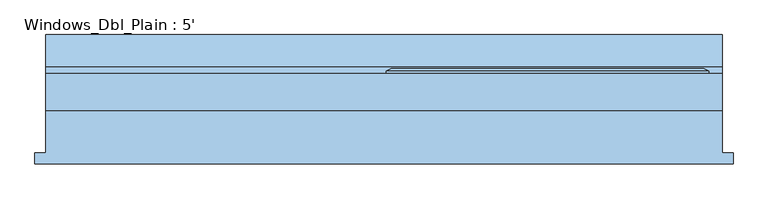
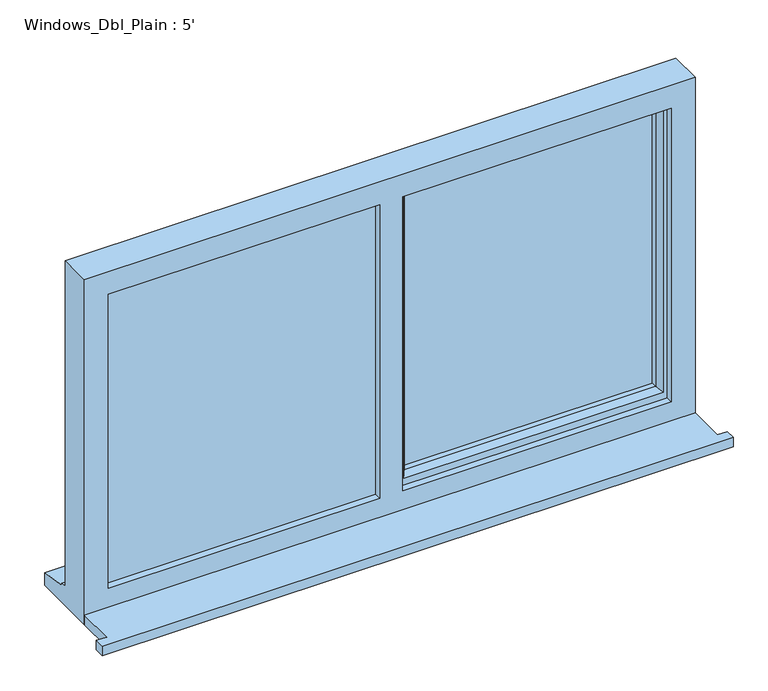
"""IFC4 building model written with IfcOpenShell, lengths in millimetres: window geometry, Windows_Dbl_Plain : 5'."""

from ifc_helpers import new_model, si_unit, frame, origin, place, context, project, spatial, polyline, outline, extrude, faceted_brep, source, transform, mapped, element, save


def windows_dbl_plain_5_e9a2d570(model_context):
    return source(origin(), model_context, "Body", "SolidModel", [
        extrude(outline(polyline([(-1072.0, -130.8434322), (-1072.0, -105.8434322), (-1047.0, -105.8434322), (-1047.0, -10.2434322), (477.0, -10.2434322), (477.0, -105.8434322), (502.0, -105.8434322), (502.0, -130.8434322), (-1072.0, -130.8434322)])), frame((0.0, 0.0, 1200.0), z_axis=(0.0, 0.0, 1.0), x_axis=(1.0, 0.0, 0.0)), (0.0, 0.0, 1.0), 25.0),
        faceted_brep([(-280.0, 72.7565678, 2080.0), (-280.0, 78.5300705, 2080.0), (-280.0, 78.5300705, 1253.0), (-280.0, 72.7565678, 1253.0), (-270.0, 7.7565678, 2070.0), (-270.0, 72.7565678, 2070.0), (-270.0, 72.7565678, 1263.0), (-270.0, 7.7565678, 1263.0), (-230.0, 22.2494677, 2030.0), (-240.1480377, 7.7565678, 2040.1480377), (-240.1480377, 7.7565678, 1292.8519623), (-230.0, 22.2494677, 1303.0), (-230.0, 36.7565678, 2030.0), (-230.0, 36.7565678, 1303.0), (-240.0, 60.7565678, 2040.0), (-240.0, 36.7565678, 2040.0), (-240.0, 36.7565678, 1293.0), (-240.0, 60.7565678, 1293.0), (-230.0, 78.5300705, 2030.0), (-230.0, 60.7565678, 2030.0), (-230.0, 60.7565678, 1303.0), (-230.0, 78.5300705, 1303.0), (-247.4457548, 84.3035732, 2047.4457548), (-247.4457548, 84.3035732, 1285.5542452), (-269.2153903, 84.3035732, 2069.2153903), (-269.2153903, 84.3035732, 1263.7846097), (447.0, 78.5300705, 1253.0), (447.0, 72.7565678, 1253.0), (437.0, 72.7565678, 1263.0), (437.0, 7.7565678, 1263.0), (407.1480377, 7.7565678, 1292.8519623), (397.0, 22.2494677, 1303.0), (397.0, 36.7565678, 1303.0), (407.0, 36.7565678, 1293.0), (407.0, 60.7565678, 1293.0), (397.0, 60.7565678, 1303.0), (397.0, 78.5300705, 1303.0), (414.4457548, 84.3035732, 1285.5542452), (436.2153903, 84.3035732, 1263.7846097), (447.0, 78.5300705, 2080.0), (447.0, 72.7565678, 2080.0), (437.0, 72.7565678, 2070.0), (437.0, 7.7565678, 2070.0), (407.1480377, 7.7565678, 2040.1480377), (397.0, 22.2494677, 2030.0), (397.0, 36.7565678, 2030.0), (407.0, 36.7565678, 2040.0), (407.0, 60.7565678, 2040.0), (397.0, 60.7565678, 2030.0), (397.0, 78.5300705, 2030.0), (414.4457548, 84.3035732, 2047.4457548), (436.2153903, 84.3035732, 2069.2153903)], [[[0, 1, 2, 3]], [[4, 5, 6, 7]], [[8, 9, 10, 11]], [[12, 8, 11, 13]], [[14, 15, 16, 17]], [[18, 19, 20, 21]], [[22, 18, 21, 23]], [[1, 24, 25, 2]], [[3, 2, 26, 27]], [[7, 6, 28, 29]], [[11, 10, 30, 31]], [[13, 11, 31, 32]], [[17, 16, 33, 34]], [[21, 20, 35, 36]], [[23, 21, 36, 37]], [[2, 25, 38, 26]], [[27, 26, 39, 40]], [[29, 28, 41, 42]], [[31, 30, 43, 44]], [[32, 31, 44, 45]], [[34, 33, 46, 47]], [[36, 35, 48, 49]], [[37, 36, 49, 50]], [[26, 38, 51, 39]], [[40, 39, 1, 0]], [[3, 27, 40, 0], [5, 41, 28, 6]], [[42, 41, 5, 4]], [[7, 29, 42, 4], [9, 43, 30, 10]], [[44, 43, 9, 8]], [[45, 44, 8, 12]], [[15, 46, 33, 16], [13, 32, 45, 12]], [[47, 46, 15, 14]], [[17, 34, 47, 14], [19, 48, 35, 20]], [[49, 48, 19, 18]], [[50, 49, 18, 22]], [[24, 51, 38, 25], [23, 37, 50, 22]], [[39, 51, 24, 1]]]),
        extrude(outline(polyline([(2050.0, -310.0), (2070.0, -310.0), (2070.0, -1007.0), (1263.0, -1007.0), (1263.0, -310.0), (1283.0, -310.0), (1283.0, -987.0), (2050.0, -987.0), (2050.0, -310.0)])), frame((0.0, 31.7565678, 0.0), z_axis=(0.0, 1.0, 0.0), x_axis=(0.0, 0.0, 1.0)), (0.0, 0.0, 1.0), 41.0),
        faceted_brep([(477.0, -10.2434322, 2110.0), (-1047.0, -10.2434322, 2110.0), (-1047.0, -10.2434322, 1200.0), (477.0, -10.2434322, 1200.0), (417.0, -10.2434322, 2050.0), (417.0, -10.2434322, 1275.0), (-252.0, -10.2434322, 1275.0), (-252.0, -10.2434322, 2050.0), (-310.0, -10.2434322, 2050.0), (-310.0, -10.2434322, 1275.0), (-987.0, -10.2434322, 1275.0), (-987.0, -10.2434322, 2050.0), (-1047.0, 72.7565678, 2110.0), (-1047.0, 72.7565678, 1251.0), (-1047.0, 87.7565678, 1249.68767), (-1047.0, 87.7565678, 1244.7449676), (-1047.0, 160.2565678, 1233.8088847), (-1047.0, 160.2565678, 1200.0), (477.0, 72.7565678, 2110.0), (477.0, 72.7565678, 1251.0), (-1007.0, 72.7565678, 2070.0), (-1007.0, 72.7565678, 1263.0), (-310.0, 72.7565678, 1263.0), (-310.0, 72.7565678, 2070.0), (-270.0, 72.7565678, 2070.0), (-270.0, 72.7565678, 1263.0), (437.0, 72.7565678, 1263.0), (437.0, 72.7565678, 2070.0), (-1007.0, 7.7565678, 2070.0), (-1007.0, 7.7565678, 1263.0), (-300.0, 7.7565678, 2070.0), (-300.0, 7.7565678, 1263.0), (-310.0, 7.7565678, 2050.0), (-987.0, 7.7565678, 2050.0), (-987.0, 7.7565678, 1275.0), (-310.0, 7.7565678, 1275.0), (-270.0, 7.7565678, 2070.0), (437.0, 7.7565678, 2070.0), (437.0, 7.7565678, 1263.0), (-270.0, 7.7565678, 1263.0), (417.0, 7.7565678, 2050.0), (-252.0, 7.7565678, 2050.0), (-252.0, 7.7565678, 1275.0), (417.0, 7.7565678, 1275.0), (-310.0, 31.7565678, 2070.0), (-300.0, 31.7565678, 2070.0), (477.0, 160.2565678, 1200.0), (477.0, 160.2565678, 1233.8088847), (477.0, 87.7565678, 1244.7449676), (477.0, 87.7565678, 1249.68767), (-300.0, 31.7565678, 1263.0), (-310.0, 31.7565678, 1263.0)], [[[0, 1, 2, 3], [4, 5, 6, 7], [8, 9, 10, 11]], [[2, 1, 12, 13, 14, 15, 16, 17]], [[13, 12, 18, 19], [20, 21, 22, 23], [24, 25, 26, 27]], [[21, 20, 28, 29]], [[28, 30, 31, 29], [32, 33, 34, 35]], [[36, 37, 38, 39], [40, 41, 42, 43]], [[33, 11, 10, 34]], [[1, 0, 18, 12]], [[28, 20, 23, 44, 45, 30]], [[27, 37, 36, 24]], [[11, 33, 32, 8]], [[40, 4, 7, 41]], [[19, 18, 0, 3, 46, 47, 48, 49]], [[27, 26, 38, 37]], [[4, 40, 43, 5]], [[45, 50, 31, 30]], [[50, 45, 44, 51]], [[51, 44, 23, 22]], [[25, 24, 36, 39]], [[41, 7, 6, 42]], [[8, 32, 35, 9]], [[46, 3, 2, 17]], [[47, 46, 17, 16]], [[48, 47, 16, 15]], [[49, 48, 15, 14]], [[19, 49, 14, 13]], [[22, 21, 29, 31, 50, 51]], [[26, 25, 39, 38]], [[6, 5, 43, 42]], [[35, 34, 10, 9]]]),
        extrude(outline(polyline([(-1007.0, 31.7565678), (-300.0, 31.7565678), (-300.0, 7.7565678), (-1007.0, 7.7565678), (-1007.0, 31.7565678)])), frame((0.0, 0.0, 1263.0), z_axis=(0.0, 0.0, 1.0), x_axis=(1.0, 0.0, 0.0)), (0.0, 0.0, 1.0), 807.0),
        extrude(outline(polyline([(407.0, 36.7565678), (-240.0, 36.7565678), (-240.0, 60.7565678), (407.0, 60.7565678), (407.0, 36.7565678)])), frame((0.0, 0.0, 1293.0), z_axis=(0.0, 0.0, 1.0), x_axis=(1.0, 0.0, 0.0)), (0.0, 0.0, 1.0), 747.0),
    ])


if __name__ == "__main__":
    model = new_model("IFC4")
    model_context = context("Model", 3, world=origin())
    ifc_project = project(units=[si_unit("LENGTHUNIT", "METRE", prefix="MILLI")], contexts=[model_context])
    site = spatial("IfcSite", under=ifc_project)
    building = spatial("IfcBuilding", under=site)
    placement = place(None, origin())
    windows_dbl_plain_5_shape = windows_dbl_plain_5_e9a2d570(model_context)
    element("IfcWindow", 1, ObjectType="Windows_Dbl_Plain : 5'", at=placement, inside=building, context=model_context, shape_type="MappedRepresentation", body=[
        mapped(windows_dbl_plain_5_shape, transform((0.0, 0.0, 0.0), x_axis=(1.0, 0.0, 0.0), y_axis=(0.0, 1.0, 0.0), z_axis=(0.0, 0.0, 1.0))),
    ])
    save(model, "model.ifc")

# Revit data of these elements
# Type "Windows_Dbl_Plain : 5'"
#   Type Mark = "58"
#   Operation = "DoublePanelVertical"
#   Construction Type Id = "GSP4R"
#   Manufacturer = "Revit"
#   Keynote = "L10"
#   Analytic Construction = "1/8 in Pilkington single glazing"
#   Wrap Layers (Ext) from Ext = 0.336286 ft
#   Wrap Layers (Int) from Ext = 0.582349 ft
#   Window Board Projection = 0.082021 ft
#   Window Board Extension = 0.082021 ft
#   Visual Light Transmittance = 0.9
#   Solar Heat Gain Coefficient = 0.78
#   Rough Width = 5.0 ft
#   Rough Height = 2.985564 ft
#   Height = 2.985564 ft
#   Width = 5.0 ft
#   Heat Transfer Coefficient (U) = 3.6886 W/(m²·K)
#   Glazing Thickness = 0.07874 ft
#   FrameOffset - External = 0.164042 ft
#   Frame Depth = 0.213255 ft
#   Default Head Height = 6.922572 ft
#   Cill Depth = 0.287073 ft
#   Cavity Closer Width = 0.164042 ft
#   Cavity Closer Offset from Ext = 0.336286 ft
#   Cavity Closer Depth = 0.278871 ft
#   Vis - Cavity Closers = yes
#   Define Thermal Properties by = 1
#   Material Trim = Window Frame
#   Material Glass = Glass
#   Material Frame = Window Frame
#   Wall Closure = (empty or 0)
# Element 1 (IfcWindow, "Windows_Dbl_Plain : 5'")
#   Materials on its faces: "Window Frame", "Glass"
# Materials
#   "Window Frame": colour RGB 249 249 249, transparency 0, Keynote = "L10", Cost = 0
#   "Glass": class "Glass", colour RGB 0 128 192, transparency 0.9, Description = "Soda Lime Glass", Cost = 0
